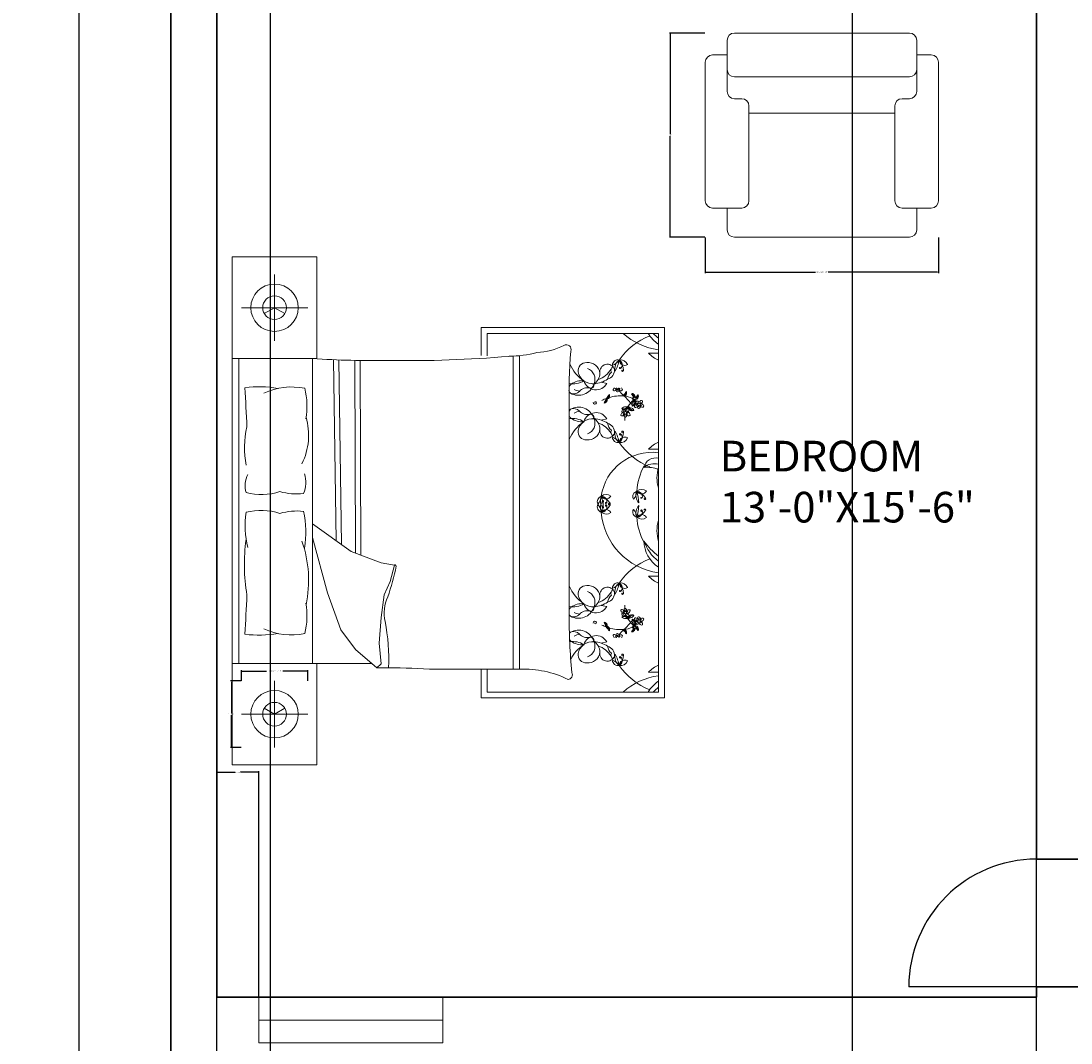
# Model space of a CAD drawing. Units: inches. Extents: x -10 to 502, y -868 to 56.
# Tile 10 of 14: x 6 to 211, y -264 to -64. Entities that reach past the tile are written whole.
import ezdxf

# ---------------------------------------------------------------- set-up
doc = ezdxf.new("R2010")
doc.units = ezdxf.units.IN
doc.header["$MEASUREMENT"] = 0
for name, color, linetype, lineweight in [('A-ANNO-DIMS', 2, 'Continuous', 18), ('A-AREA-IDEN', 7, 'Continuous', 18), ('A-DOOR', 4, 'Continuous', 25), ('A-FURN', 8, 'Continuous', 13), ('A-GLAZ', 162, 'Continuous', 18), ('A-WALL', 7, 'Continuous', 35)]:
    doc.layers.add(name, color=color, linetype=linetype, lineweight=lineweight)
doc.styles.get("Standard").update_dxf_attribs({"font": 'arial.ttf'})
doc.dimstyles.get("Standard").update_dxf_attribs({"dimtxt": 0.18, "dimasz": 0.18, "dimexe": 0.18, "dimexo": 0.0625, "dimgap": 0.09, "dimtad": 0, "dimtih": 1, "dimtoh": 1, "dimdec": 0, "dimzin": 0, "dimdsep": 46, "dimlunit": 3, "dimtxsty": 'Standard', "dimcen": 0.09, "dimadec": 0, "dimazin": 0, "dimtfac": 1, "dimtdec": 0, "dimtofl": 0, "dimtmove": 0, "dimatfit": 3, "dimfxl": 1, "dimtolj": 1, "dimtzin": 0, "dimarcsym": 0})

# ---------------------------------------------------------------- blocks, each defined once
blk = doc.blocks.new('*D2')
at = {"layer": 'A-ANNO-DIMS', "color": 0, "lineweight": -2, "transparency": 16777216}
for p, q in [((34.89, 12.15), (16.75, 12.15)), ((16.93, 11.97), (16.93, -376.2)), ((16.93, -770.67), (16.93, -382.51)), ((34.89, -770.85), (16.75, -770.85))]:
    blk.add_line(p, q, dxfattribs=at)
at = {"layer": 'A-ANNO-DIMS', "color": 0, "transparency": 16777216}
for points in [[(16.9, 11.97), (16.96, 11.97), (16.93, 12.15)], [(16.9, -770.67), (16.96, -770.67), (16.93, -770.85)]]:
    blk.add_solid(points, dxfattribs=at)
at = {"layer": 'Defpoints', "color": 0, "transparency": 16777216}
for p in [(34.95, 12.15), (16.93, -770.85), (34.95, -770.85)]:
    blk.add_point(p, dxfattribs=at)
at = {"layer": 'A-ANNO-DIMS', "color": 0, "transparency": 16777216, "insert": (16.93, -379.35), "char_height": 6, "attachment_point": 5}
blk.add_mtext('\\A1;65\'-3"', dxfattribs=at)
blk = doc.blocks.new('A$C14264F02')
at = {"color": 0}
for p, q in [((0.1, 0.7), (0.7, 0.7)), ((0.1, 0.7), (0.7, 0.7)), ((0.075, 0.625), (0.075, 0.675)), ((0.075, 0.625), (0.075, 0.675)), ((0.725, 0.675), (0.725, 0.575)), ((0.725, 0.675), (0.725, 0.625)), ((0.075, 0.625), (0.025, 0.625)), ((0.025, 0.625), (0.075, 0.625)), ((0.075, 0.575), (0.075, 0.625)), ((0.725, 0.625), (0.775, 0.625)), ((0.725, 0.625), (0.775, 0.625)), ((0, 0.125), (0, 0.6)), ((0, 0.125), (0, 0.6)), ((0.8, 0.6), (0.8, 0.125)), ((0.8, 0.6), (0.8, 0.125)), ((0.075, 0.575), (0.075, 0.5)), ((0.7, 0.55), (0.1, 0.55)), ((0.725, 0.5), (0.725, 0.575)), ((0.1, 0.475), (0.125, 0.475)), ((0.675, 0.475), (0.7, 0.475)), ((0.15, 0.45), (0.15, 0.125)), ((0.65, 0.125), (0.65, 0.45)), ((0.65, 0.425), (0.15, 0.425)), ((0.075, 0.1), (0.025, 0.1)), ((0.075, 0.1), (0.025, 0.1)), ((0.075, 0.025), (0.075, 0.1)), ((0.125, 0.1), (0.075, 0.1)), ((0.775, 0.1), (0.675, 0.1)), ((0.775, 0.1), (0.725, 0.1)), ((0.725, 0.1), (0.725, 0.025)), ((0.7, 0), (0.1, 0))]:
    blk.add_line(p, q, dxfattribs=at)
for centre, start, end in [((0.1, 0.675), 90, 180), ((0.1, 0.675), 90, 180), ((0.7, 0.675), 0, 90), ((0.7, 0.675), 360, 90), ((0.025, 0.6), 90, 180), ((0.025, 0.6), 90, 180), ((0.775, 0.6), 360, 90), ((0.775, 0.6), 0, 90), ((0.1, 0.575), 180, 270), ((0.7, 0.575), 270, 0), ((0.1, 0.5), 180, 270), ((0.125, 0.45), 0, 90), ((0.675, 0.45), 90, 180), ((0.7, 0.5), 270, 360), ((0.025, 0.125), 180, 270), ((0.025, 0.125), 180, 270), ((0.125, 0.125), 270, 360), ((0.675, 0.125), 180, 270), ((0.775, 0.125), 270, 360), ((0.775, 0.125), 270, 360), ((0.1, 0.025), 180, 270), ((0.7, 0.025), 270, 360)]:
    blk.add_arc(centre, 0.025, start, end, dxfattribs=at)
blk = doc.blocks.new('WIN-36IN')
for p, q in [((0, 9), (36, 9)), ((0, 0), (0, 9)), ((36, 9), (36, 0)), ((0, 4.5), (36, 4.5)), ((36, 0), (0, 0))]:
    blk.add_line(p, q)
blk = doc.blocks.new('DOOR-SWING-25IN')
blk.add_line((25, 0), (0, 0))
blk.add_arc((25, 0), 25, 90, 180)
blk = doc.blocks.new('LAMP-BEDSIDE-SMALL')
for p, q in [((6.5, 0), (6.5, 13)), ((13, 6.5), (0, 6.5))]:
    blk.add_line(p, q)
for points in [[(6.5, 6.5), (4.49, 5.34)], [(6.5, 6.5), (8.51, 5.34)]]:
    blk.add_lwpolyline(points)
for radius in [4.64, 2.32]:
    blk.add_circle((6.5, 6.5), radius)
blk = doc.blocks.new('*D35')
at = {"layer": 'A-ANNO-DIMS', "color": 0, "lineweight": -2, "transparency": 16777216}
for p, q in [((139.59, -106.11), (139.59, -113.08)), ((185.27, -106.11), (185.27, -113.08)), ((139.77, -112.9), (161.18, -112.9)), ((185.09, -112.9), (163.68, -112.9))]:
    blk.add_line(p, q, dxfattribs=at)
at = {"layer": 'A-ANNO-DIMS', "color": 0, "transparency": 16777216}
for points in [[(139.77, -112.87), (139.77, -112.93), (139.59, -112.9)], [(185.09, -112.87), (185.09, -112.93), (185.27, -112.9)]]:
    blk.add_solid(points, dxfattribs=at)
at = {"layer": 'Defpoints', "color": 0, "transparency": 16777216}
for p in [(139.59, -106.05), (185.27, -106.05), (139.59, -112.9)]:
    blk.add_point(p, dxfattribs=at)
at = {"layer": 'A-ANNO-DIMS', "color": 0, "transparency": 16777216, "insert": (162.43, -112.9), "char_height": 0.18, "attachment_point": 5}
blk.add_mtext('\\A1;ARMCHAIR 3\'-9 1/2"', dxfattribs=at)
blk = doc.blocks.new('*D36')
at = {"layer": 'A-ANNO-DIMS', "color": 0, "lineweight": -2, "transparency": 16777216}
for p, q in [((139.53, -66.07), (132.56, -66.07)), ((132.74, -66.25), (132.74, -85.88)), ((132.74, -105.87), (132.74, -86.24)), ((139.53, -106.05), (132.56, -106.05))]:
    blk.add_line(p, q, dxfattribs=at)
at = {"layer": 'A-ANNO-DIMS', "color": 0, "transparency": 16777216}
for points in [[(132.71, -66.25), (132.77, -66.25), (132.74, -66.07)], [(132.71, -105.87), (132.77, -105.87), (132.74, -106.05)]]:
    blk.add_solid(points, dxfattribs=at)
at = {"layer": 'Defpoints', "color": 0, "transparency": 16777216}
for p in [(132.74, -66.07), (139.59, -66.07), (139.59, -106.05)]:
    blk.add_point(p, dxfattribs=at)
at = {"layer": 'A-ANNO-DIMS', "color": 0, "transparency": 16777216, "insert": (132.74, -86.06), "char_height": 0.18, "attachment_point": 5}
blk.add_mtext('\\A1;3\'-4"', dxfattribs=at)
blk = doc.blocks.new('*D43')
at = {"layer": 'A-ANNO-DIMS', "color": 0, "lineweight": -2, "transparency": 16777216}
for p, q in [((48.76, -192.9), (48.76, -190.83)), ((48.94, -191.01), (53.66, -191.01)), ((61.58, -191.01), (56.86, -191.01)), ((61.76, -192.9), (61.76, -190.83))]:
    blk.add_line(p, q, dxfattribs=at)
at = {"layer": 'A-ANNO-DIMS', "color": 0, "transparency": 16777216}
for points in [[(48.94, -190.98), (48.94, -191.04), (48.76, -191.01)], [(61.58, -190.98), (61.58, -191.04), (61.76, -191.01)]]:
    blk.add_solid(points, dxfattribs=at)
at = {"layer": 'Defpoints', "color": 0, "transparency": 16777216}
for p in [(48.76, -191.01), (48.76, -192.96), (61.76, -192.96)]:
    blk.add_point(p, dxfattribs=at)
at = {"layer": 'A-ANNO-DIMS', "color": 0, "transparency": 16777216, "insert": (55.26, -191.01), "char_height": 0.18, "attachment_point": 5}
blk.add_mtext('\\A1;BEDSIDE LAMP 1\'-1" TYP.', dxfattribs=at)
blk = doc.blocks.new('*D44')
at = {"layer": 'A-ANNO-DIMS', "color": 0, "lineweight": -2, "transparency": 16777216}
for p, q in [((48.7, -192.96), (46.63, -192.96)), ((46.81, -193.14), (46.81, -199.28)), ((46.81, -205.78), (46.81, -199.64)), ((48.7, -205.96), (46.63, -205.96))]:
    blk.add_line(p, q, dxfattribs=at)
at = {"layer": 'A-ANNO-DIMS', "color": 0, "transparency": 16777216}
for points in [[(46.78, -193.14), (46.84, -193.14), (46.81, -192.96)], [(46.78, -205.78), (46.84, -205.78), (46.81, -205.96)]]:
    blk.add_solid(points, dxfattribs=at)
at = {"layer": 'Defpoints', "color": 0, "transparency": 16777216}
for p in [(48.76, -192.96), (46.81, -205.96), (48.76, -205.96)]:
    blk.add_point(p, dxfattribs=at)
at = {"layer": 'A-ANNO-DIMS', "color": 0, "transparency": 16777216, "insert": (46.81, -199.46), "char_height": 0.18, "attachment_point": 5}
blk.add_mtext('\\A1;1\'-1" TYP.', dxfattribs=at)
blk = doc.blocks.new('*D60')
at = {"layer": 'A-ANNO-DIMS', "color": 0, "lineweight": -2, "transparency": 16777216}
for p, q in [((168.45, -332.79), (168.45, 56.38)), ((168.63, 56.2), (186.12, 56.2)), ((204.27, 56.2), (186.78, 56.2)), ((204.45, -332.79), (204.45, 56.38))]:
    blk.add_line(p, q, dxfattribs=at)
at = {"layer": 'A-ANNO-DIMS', "color": 0, "transparency": 16777216}
for points in [[(168.63, 56.23), (168.63, 56.17), (168.45, 56.2)], [(204.27, 56.23), (204.27, 56.17), (204.45, 56.2)]]:
    blk.add_solid(points, dxfattribs=at)
at = {"layer": 'Defpoints', "color": 0, "transparency": 16777216}
for p in [(204.45, 56.2), (168.45, -332.85), (204.45, -332.85)]:
    blk.add_point(p, dxfattribs=at)
at = {"layer": 'A-ANNO-DIMS', "color": 0, "transparency": 16777216, "insert": (186.45, 56.2), "char_height": 0.18, "attachment_point": 5}
blk.add_mtext('\\A1;3\'-0"', dxfattribs=at)
blk = doc.blocks.new('*D61')
at = {"layer": 'A-ANNO-DIMS', "color": 0, "lineweight": -2, "transparency": 16777216}
for p, q in [((43.95, -254.79), (43.95, -210.62)), ((44.13, -210.8), (47.54, -210.8)), ((52.02, -210.8), (48.61, -210.8)), ((52.2, -254.79), (52.2, -210.62))]:
    blk.add_line(p, q, dxfattribs=at)
at = {"layer": 'A-ANNO-DIMS', "color": 0, "transparency": 16777216}
for points in [[(44.13, -210.77), (44.13, -210.83), (43.95, -210.8)], [(52.02, -210.77), (52.02, -210.83), (52.2, -210.8)]]:
    blk.add_solid(points, dxfattribs=at)
at = {"layer": 'Defpoints', "color": 0, "transparency": 16777216}
for p in [(52.2, -210.8), (43.95, -254.85), (52.2, -254.85)]:
    blk.add_point(p, dxfattribs=at)
at = {"layer": 'A-ANNO-DIMS', "color": 0, "transparency": 16777216, "insert": (48.08, -210.8), "char_height": 0.18, "attachment_point": 5}
blk.add_mtext('\\A1;0\'-8 1/2"', dxfattribs=at)
blk = doc.blocks.new('*D64')
at = {"layer": 'A-ANNO-DIMS', "color": 0, "lineweight": -2, "transparency": 16777216}
for p, q in [((43.95, -332.79), (43.95, 56.38)), ((44.13, 56.2), (48.59, 56.2)), ((54.27, 56.2), (49.81, 56.2)), ((54.45, -332.79), (54.45, 56.38))]:
    blk.add_line(p, q, dxfattribs=at)
at = {"layer": 'A-ANNO-DIMS', "color": 0, "transparency": 16777216}
for points in [[(44.13, 56.23), (44.13, 56.17), (43.95, 56.2)], [(54.27, 56.23), (54.27, 56.17), (54.45, 56.2)]]:
    blk.add_solid(points, dxfattribs=at)
at = {"layer": 'Defpoints', "color": 0, "transparency": 16777216}
for p in [(54.45, 56.2), (43.95, -332.85), (54.45, -332.85)]:
    blk.add_point(p, dxfattribs=at)
at = {"layer": 'A-ANNO-DIMS', "color": 0, "transparency": 16777216, "insert": (49.2, 56.2), "char_height": 0.18, "attachment_point": 5}
blk.add_mtext('\\A1;0\'-10 1/2"', dxfattribs=at)

msp = doc.modelspace()

# ---------------------------------------------------------------- linework, layer by layer
at = {"layer": 'A-FURN'}
for p, q in [((46.97, -209.41), (46.97, -109.91)), ((95.74, -129.25), (95.74, -123.74)), ((95.74, -123.74), (131.59, -123.74)), ((96.9, -124.89), (96.9, -129.28)), ((130.43, -124.89), (96.9, -124.89)), ((130.43, -195.12), (130.43, -124.89)), ((131.59, -123.74), (131.59, -196.28)), ((101.95, -129.36), (101.95, -190.66)), ((103.19, -129.26), (103.19, -190.66)), ((48.24, -129.81), (48.24, -189.51)), ((62.69, -189.51), (62.69, -129.81)), ((66.82, -130.08), (67.32, -165.5)), ((67.85, -130.11), (68.36, -166.25)), ((70.98, -130.17), (71.13, -167.95)), ((72, -130.16), (72.16, -168.34)), ((120.35, -134.69), (119.22, -134.47)), ((112.96, -139.46), (112.96, -179.86)), ((120.35, -141.65), (119.22, -141.87)), ((62.69, -162.18), (70.28, -167.63)), ((65.65, -175.69), (62.69, -164.84)), ((70.28, -167.63), (76.12, -169.84)), ((76.12, -169.84), (78.74, -170.25)), ((78.74, -170.25), (77.93, -173.47)), ((77.93, -173.47), (76.73, -176.09)), ((68.27, -182.94), (65.65, -175.69)), ((76.73, -176.09), (76.12, -180.53)), ((120.35, -178.37), (119.22, -178.15)), ((76.12, -180.53), (75.72, -185.56)), ((71.09, -186.77), (68.27, -182.94)), ((75.32, -190.4), (71.09, -186.77)), ((75.72, -185.56), (76.12, -189.6)), ((120.35, -185.32), (119.22, -185.54)), ((46.97, -189.51), (74.28, -189.51)), ((76.12, -189.6), (75.32, -190.4)), ((95.74, -196.28), (95.74, -190.65)), ((96.9, -190.65), (96.9, -195.12)), ((96.9, -195.12), (130.43, -195.12)), ((131.59, -196.28), (95.74, -196.28))]:
    msp.add_line(p, q, dxfattribs=at)
for points in [[(46.97, -129.81), (63.55, -129.81), (63.55, -109.91), (46.97, -109.91)], [(63.55, -189.51), (63.55, -209.41), (46.97, -209.41)]]:
    msp.add_lwpolyline(points, dxfattribs=at)
for points in [[(101.17, -129.38, 0.056112), (106.64, -128.66, 0.095341), (111.91, -127.26)], [(49.45, -135.52, -0.074897), (55.95, -135.65, 0.472817)], [(56.31, -155.88, -0.14099), (49.68, -156.08, -0.235245)], [(56.31, -160.13, 0.14099), (49.68, -159.93, 0.235245)], [(49.45, -183.8, 0.074897), (55.95, -183.67, -0.472817)], [(84.43, -190.61, 0.001242), (103.31, -190.66, -0.127202), (112.72, -192.65)]]:
    msp.add_lwpolyline(points, format="xyb", dxfattribs=at)
for centre in [(126.62, -138.79), (123.95, -140.44), (123.95, -179.57), (126.62, -181.23)]:
    msp.add_circle(centre, 0.253, dxfattribs=at)
for centre, radius, start, end in [((133.47, -137.45), 12.99, 111.4092, 145.6135), ((132.18, -115.22), 12.99, 228.1144, 262.255), ((133.92, -121.73), 6.33, 209.8884, 236.5383), ((135.11, -119.46), 7.89, 223.5186, 233.6964), ((112.42, -128.02), 0.907, 336.5219, 123.8264), ((81.35, 102.99), 233.22, 269.1145, 274.8735), ((209.74, -136.41), 96.82, 175.2402, 181.8035), ((132.46, -125.28), 5.28, 221.0454, 247.4453), ((129.62, -110.81), 17.98, 266.3481, 272.5919), ((74.85, 48.57), 178.79, 266.1, 270.9282), ((119.97, -127.89), 7.53, 203.6453, 236.3329), ((116.35, -132.28), 1.68, 88.9462, 185.5144), ((116.6, -132.97), 2.38, 7.1143, 95.0551), ((120.43, -132.42), 1.49, 19.1312, 189.736), ((122.04, -132.11), 0.915, 126.7319, 206.0245), ((122.49, -131.15), 1.08, 76.272, 177.0484), ((120.85, -128.95), 2.22, 284.7031, 328.6173), ((123.95, -131.77), 2.05, 125.7657, 194.5347), ((113.87, -128.14), 9.09, 332.8176, 347.4827), ((123.05, -131.52), 1.44, 20.9613, 102.2885), ((123.83, -130.08), 1.09, 181.7131, 301.5367), ((120.27, -132.27), 3.29, 2.0648, 41.1598), ((122.25, -131.05), 1.06, 316.2238, 62.3173), ((117.6, -131.76), 2.99, 193.079, 274.7067), ((115.69, -133.9), 2.31, 338.5779, 68.4181), ((116.07, -132.55), 2.89, 305.9599, 357.6409), ((117.14, -129.46), 4.7, 288.2955, 328.7386), ((119.98, -132.06), 1.86, 285.6955, 4.031), ((122.46, -134.07), 1.99, 128.4175, 173.8338), ((122.87, -131.67), 0.0847, 20.2667, 316.2271), ((123.4, -132.16), 0.161, 168.5166, 2.0648), ((123.31, -132.14), 0.0784, 52.0591, 168.5166), ((-897.48, -190.37), 948.52, 2.85022, 3.31479), ((58.56, -148.2), 12.82, 78.2417, 114.8684), ((48.28, -139.07), 13.33, 348.9631, 14.8961), ((114.06, -135.76), 1.2, 127.675, 162.5814), ((113.7, -130.65), 4.12, 259.249, 301.1782), ((114.77, -133.84), 3.17, 240.8249, 340.7178), ((115.49, -137.98), 3.84, 85.2696, 124.215), ((116.47, -137.59), 2.04, 74.8529, 138.4347), ((118.2, -133.46), 2.47, 196.8663, 330.0915), ((117.16, -135.03), 0.618, 254.8529, 12.6959), ((115.49, -137.98), 3.84, 53.6555, 57.2989), ((117.52, -129.41), 5.34, 273.4924, 303.7117), ((122.05, -135.88), 0.423, 127.3642, 168.4363), ((122.21, -135.83), 0.242, 88.1325, 178.8919), ((122.45, -135.53), 0.253, 183.2768, 356.7232), ((122.36, -136.33), 0.769, 42.3896, 66.5724), ((122.91, -135.88), 0.418, 10.9597, 52.2379), ((114.06, -135.76), 1.2, 196.6343, 225.5483), ((113.83, -135.25), 1.49, 246.1646, 318.4347), ((115.35, -133.37), 2.86, 240.0851, 262.564), ((123.11, -145.35), 8.24, 110.1059, 116.9968), ((120.29, -137.93), 0.203, 83.9457, 185.6216), ((119.48, -137.74), 0.834, 328.836, 0.8141), ((119.91, -137.98), 0.478, 306.5232, 32.4668), ((120.48, -137.61), 0.203, 112.5583, 214.2343), ((120.34, -137.25), 0.478, 265.7131, 351.6568), ((119.93, -136.98), 0.834, 297.3659, 329.344), ((119.29, -136.27), 1.6, 313.6929, 321.7899), ((121.06, -137.36), 0.522, 115.5379, 168.6744), ((119.29, -136.61), 1.57, 329.344, 349.7412), ((123.11, -145.35), 8.24, 86.1723, 106.4158), ((118.03, -136.97), 2.81, 352.8698, 1.6736), ((121.75, -135.96), 0.196, 125.0752, 284.7644), ((121.72, -135.54), 0.609, 277.4968, 341.2737), ((122.69, -136.08), 0.524, 136.3462, 189.6513), ((122.39, -136.13), 0.218, 189.6513, 312.3208), ((123.24, -135.98), 0.83, 164.2829, 186.9148), ((122.26, -135.99), 0.415, 312.3208, 40.2111), ((123.14, -135.52), 0.589, 201.6382, 274.947), ((130.12, -130.24), 9.45, 217.9541, 226.8459), ((123.17, -135.92), 0.194, 274.947, 37.5263), ((123.82, -137.02), 0.203, 112.5583, 214.2343), ((123.69, -136.66), 0.478, 265.7131, 351.6568), ((123.27, -136.39), 0.834, 297.3659, 329.344), ((123.31, -141.25), 4.13, 60.7959, 85.244), ((114.52, -147.2), 13.6, 37.8256, 47.7588), ((122.64, -135.67), 1.6, 313.6929, 321.7899), ((124.41, -136.77), 0.522, 115.5379, 168.6744), ((122.64, -136.01), 1.57, 329.344, 349.7412), ((121.38, -136.38), 2.81, 352.8698, 1.6736), ((125.33, -136.94), 0.283, 33.0979, 123.1364), ((119.09, -140.93), 7.4, 31.1156, 34.8118), ((124.92, -137.43), 0.766, 2.3172, 70.5201), ((125.55, -137.62), 0.221, 135.7354, 318.1297), ((125.18, -137.26), 0.293, 315.7354, 31.1156), ((125.72, -137.61), 0.221, 68.2452, 250.6395), ((125.21, -137.34), 0.66, 352.6008, 57.1845), ((127.56, -141.77), 4.41, 111.7087, 116.2181), ((125.84, -137.19), 0.66, 252.8042, 349.6943), ((125.91, -137.14), 0.293, 248.2452, 323.6254), ((125.65, -136.96), 0.766, 291.7087, 3.0299), ((120.18, -132.92), 7.4, 323.6254, 327.3216), ((126.25, -137.15), 0.283, 325.6077, 55.6462), ((114.06, -140.59), 1.2, 134.4517, 156.7144), ((114.77, -142.5), 3.17, 19.2822, 119.1751), ((113.83, -141.09), 1.49, 41.5653, 113.8354), ((117.98, -138.44), 0.312, 169.5864, 349.5616), ((118.1, -138.46), 0.192, 349.5616, 167.2949), ((120.34, -138.56), 0.522, 129.5056, 182.6421), ((118.84, -137.35), 1.57, 308.4388, 328.836), ((118.57, -136.07), 2.81, 296.5064, 305.3102), ((118.55, -137.52), 1.6, 336.3901, 344.4871), ((123.57, -138.5), 1.16, 253.6301, 325.4631), ((123.9, -140.11), 0.817, 82.0748, 142.6895), ((123.81, -138.98), 0.839, 228.342, 274.9894), ((123.83, -139.12), 0.702, 273.8774, 357.1501), ((124.72, -140.38), 0.799, 121.9501, 165.2442), ((124.11, -138.62), 0.68, 262.0748, 308.2393), ((124.14, -139.93), 0.5, 278.5614, 22.5914), ((128.8, -141.67), 4.96, 156.1523, 156.9499), ((124.43, -139.91), 0.251, 44.3732, 121.9501), ((125.2, -139.32), 0.702, 181.4625, 249.4747), ((128.8, -141.67), 4.96, 130.182, 149.456), ((125.08, -138.77), 0.68, 215.1128, 261.2773), ((125.63, -138.8), 1.16, 197.889, 269.722), ((124.86, -140.25), 0.817, 20.6625, 81.2773), ((126.07, -138.85), 0.817, 139.3812, 199.9959), ((124.55, -138.26), 1.16, 310.9365, 22.7695), ((125.08, -138.32), 0.839, 285.6484, 332.2957), ((124.94, -137.88), 0.68, 319.3812, 5.5456), ((123.31, -141.25), 4.13, 47.5083, 55.9967), ((125.21, -138.37), 0.702, 331.1838, 51.6792), ((125.93, -139.21), 0.196, 125.0752, 284.7644), ((126.23, -139.14), 0.423, 93.635, 168.4363), ((126.18, -138.47), 0.248, 138.2946, 276.2474), ((125.9, -138.8), 0.609, 277.4968, 341.2737), ((126.27, -138.51), 0.346, 358.5719, 143.8954), ((126.38, -139.08), 0.242, 88.1325, 178.8919), ((126.47, -138.23), 0.349, 208.8493, 269.9355), ((126.17, -138.32), 0.399, 274.2123, 318.1587), ((126.87, -139.34), 0.524, 136.3462, 189.6513), ((126.57, -139.39), 0.218, 189.6513, 312.3208), ((127.41, -139.24), 0.83, 164.2829, 186.9148), ((127.39, -138.72), 0.799, 121.9501, 165.2442), ((126.44, -139.24), 0.415, 312.3208, 40.2111), ((127.31, -138.78), 0.589, 201.6382, 274.947), ((126.84, -138.41), 0.168, 262.868, 7.094), ((126.53, -139.58), 0.769, 42.3896, 66.5724), ((126.82, -138.27), 0.5, 278.5614, 22.5914), ((127.09, -139.13), 0.418, 10.9597, 118.7804), ((127.1, -138.25), 0.251, 44.3732, 121.9501), ((127.35, -139.17), 0.194, 274.947, 37.5263), ((49.26, -144.83), 12.67, 333.8761, 16.1746), ((114.06, -140.59), 1.2, 203.2856, 232.325), ((113.7, -145.69), 4.12, 58.8218, 100.2867), ((115.49, -138.36), 3.84, 235.785, 274.7304), ((115.35, -142.98), 2.86, 97.436, 119.9149), ((117.6, -144.58), 2.99, 85.2933, 166.921), ((116.47, -138.75), 2.04, 221.5653, 285.1471), ((118.2, -142.88), 2.47, 29.9085, 163.1337), ((115.69, -142.44), 2.31, 291.5819, 21.4221), ((117.16, -141.32), 0.618, 347.3041, 105.1471), ((115.49, -138.36), 3.84, 302.7011, 306.3445), ((116.07, -143.79), 2.89, 2.3591, 54.0401), ((117.52, -146.93), 5.34, 56.2883, 86.5076), ((123.26, -140.87), 0.196, 125.0752, 284.7644), ((123.56, -140.79), 0.423, 93.635, 168.4363), ((123.51, -140.13), 0.248, 138.2946, 276.2474), ((123.23, -140.45), 0.609, 277.4968, 341.2737), ((123.6, -140.16), 0.346, 358.5719, 143.8954), ((123.71, -140.74), 0.242, 88.1325, 178.8919), ((123.8, -139.89), 0.349, 208.8493, 269.9355), ((123.5, -139.97), 0.399, 274.2123, 318.1587), ((124.2, -141), 0.524, 136.3462, 189.6513), ((123.9, -141.05), 0.218, 189.6513, 312.3208), ((128.8, -141.67), 4.96, 175.2415, 182.8929), ((124.74, -140.9), 0.83, 164.2829, 186.9148), ((123.77, -140.9), 0.415, 312.3208, 40.2111), ((124.64, -140.43), 0.589, 201.6382, 274.947), ((124.17, -140.07), 0.168, 262.868, 7.094), ((123.86, -141.24), 0.769, 42.3896, 66.5724), ((124.42, -140.79), 0.418, 10.9597, 118.7804), ((124.68, -140.83), 0.194, 274.947, 37.5263), ((125.27, -139.2), 0.839, 248.3627, 295.0101), ((66.86, -147.33), 17.49, 166.3427, 191.1841), ((119.97, -148.45), 7.53, 123.6671, 158.5059), ((116.35, -144.07), 1.68, 174.4856, 271.0538), ((116.6, -143.38), 2.38, 264.9449, 352.8857), ((117.14, -146.89), 4.7, 31.2614, 71.7045), ((120.43, -143.92), 1.49, 170.264, 340.8688), ((122.46, -142.27), 1.99, 186.1662, 231.5825), ((119.98, -144.28), 1.86, 355.969, 74.3045), ((122.04, -144.23), 0.915, 153.9755, 233.2681), ((122.49, -145.19), 1.08, 182.9516, 283.728), ((120.85, -147.39), 2.22, 31.3827, 75.2969), ((123.95, -144.57), 2.05, 165.4653, 234.2343), ((113.87, -148.21), 9.09, 12.5173, 27.1824), ((120.27, -144.07), 3.29, 318.8402, 357.9352), ((122.25, -145.29), 1.06, 297.6827, 43.7762), ((123.83, -146.27), 1.09, 58.4633, 178.2869), ((123.05, -144.83), 1.44, 257.7115, 339.0387), ((122.92, -144.66), 0.141, 43.7762, 339.7183), ((123.4, -144.19), 0.161, 357.9352, 191.4834), ((123.31, -144.2), 0.0784, 191.4834, 307.9409), ((133.47, -138.9), 12.99, 214.3865, 248.5908), ((132.46, -151.06), 5.28, 112.5547, 138.9546), ((129.62, -165.53), 17.98, 87.4081, 93.6519), ((129.18, -158.23), 10.06, 82.8636, 171.8197), ((129.88, -151.59), 2.33, 76.3898, 169.0739), ((139.14, -156.82), 12.99, 152.5854, 175.5377), ((129.56, -153.35), 2.95, 72.8609, 131.9049), ((128.27, -156.93), 5.82, 68.117, 96.6195), ((137.27, -153.18), 7.14, 162.9798, 196.4569), ((54.41, -154.71), 4.92, 153.3437, 196.1026), ((56.13, -154.05), 5.27, 335.0183, 18.5407), ((59.64, -144.15), 12.19, 254.1707, 275.9871), ((126.49, -156.84), 1.08, 106.1963, 206.9726), ((123.97, -155.75), 2.22, 314.6273, 358.5415), ((128.06, -156.65), 2.05, 155.6899, 224.4589), ((127.16, -156.87), 1.44, 50.8855, 132.2127), ((127.11, -155.24), 1.09, 211.6373, 331.4609), ((126.23, -156.87), 1.06, 346.148, 92.2415), ((125.12, -158.91), 3.29, 31.989, 71.0841), ((117.52, -158.52), 9.09, 2.7418, 17.407), ((140.95, -156.01), 10.57, 174.3643, 175.6213), ((148.19, -161.58), 18.88, 160.0972, 160.2783), ((119.53, -157.83), 1.08, 106.1963, 206.9726), ((117.01, -156.74), 2.22, 314.6273, 358.5415), ((121.1, -157.65), 2.05, 155.6899, 224.4589), ((121.1, -159.05), 2.05, 135.5411, 204.3101), ((120.2, -157.87), 1.44, 50.8855, 132.2127), ((120.15, -156.23), 1.09, 211.6373, 331.4609), ((119.27, -157.86), 1.06, 346.148, 92.2415), ((118.17, -159.91), 3.29, 31.989, 71.0841), ((110.56, -159.52), 9.09, 2.7418, 17.407), ((110.56, -157.18), 9.09, 342.593, 357.2582), ((120.11, -158.1), 0.0847, 50.1909, 346.0209), ((120.82, -158.25), 0.161, 198.4408, 31.989), ((120.74, -158.28), 0.0784, 81.9833, 198.4408), ((120.82, -158.44), 0.161, 328.011, 161.5592), ((127.07, -157.1), 0.0847, 50.1909, 346.0209), ((127.78, -157.26), 0.161, 198.4408, 31.989), ((127.7, -157.28), 0.0784, 81.9833, 198.4408), ((67.22, -162.54), 17.73, 171.5249, 193.96), ((59.64, -171.86), 12.19, 84.0129, 105.8293), ((43.85, -163.86), 17.55, 349.8617, 13.6238), ((119.53, -158.86), 1.08, 153.0274, 253.8037), ((117.01, -159.95), 2.22, 1.4585, 45.3727), ((118.17, -156.79), 3.29, 288.9159, 328.011), ((119.27, -158.84), 1.06, 267.7585, 13.852), ((120.15, -160.47), 1.09, 28.5391, 148.3627), ((120.2, -158.83), 1.44, 227.7873, 309.1145), ((132.18, -158.89), 12.99, 184.4623, 262.255), ((120.17, -158.61), 0.141, 13.852, 309.9245), ((120.74, -158.42), 0.0784, 161.5592, 278.0167), ((126.49, -159.86), 1.08, 153.0274, 253.8037), ((123.97, -160.95), 2.22, 1.4585, 45.3727), ((128.06, -160.05), 2.05, 135.5411, 204.3101), ((117.52, -158.17), 9.09, 342.593, 357.2582), ((125.12, -157.78), 3.29, 288.9159, 328.011), ((126.23, -159.83), 1.06, 267.7585, 13.852), ((127.13, -159.61), 0.141, 13.852, 309.9245), ((127.78, -159.44), 0.161, 328.011, 161.5592), ((127.7, -159.41), 0.0784, 161.5592, 278.0167), ((127.11, -161.46), 1.09, 28.5391, 148.3627), ((127.16, -159.82), 1.44, 227.7873, 309.1145), ((139.14, -159.88), 12.99, 184.4623, 207.4146), ((137.27, -163.51), 7.14, 163.5431, 197.0202), ((140.95, -160.68), 10.57, 184.3787, 185.6357), ((148.19, -155.12), 18.88, 199.7217, 199.9028), ((85.45, -170.16), 36.09, 172.2196, 189.497), ((38.8, -173.23), 23.13, 348.0397, 19.2615), ((133.92, -165.4), 6.33, 181.272, 236.5383), ((137.32, -158.98), 11.74, 214.0123, 234.053), ((135.11, -163.13), 7.89, 197.8504, 233.6964), ((41.14, -163.34), 38.59, 340.1194, 349.3383), ((78.82, -170.47), 0.24, 358.8623, 109.7536), ((133.47, -181.12), 12.99, 111.4092, 145.6135), ((129.62, -154.48), 17.98, 266.3481, 272.5919), ((132.46, -168.95), 5.28, 221.0454, 247.4453), ((119.97, -171.56), 7.53, 201.4941, 236.3329), ((116.35, -175.95), 1.68, 88.9462, 185.5144), ((116.6, -176.64), 2.38, 7.1143, 95.0551), ((120.43, -176.09), 1.49, 19.1312, 189.736), ((122.49, -174.82), 1.08, 76.272, 177.0484), ((120.85, -172.62), 2.22, 284.7031, 328.6173), ((123.95, -175.44), 2.05, 125.7657, 194.5347), ((113.87, -171.81), 9.09, 332.8176, 347.4827), ((123.05, -175.19), 1.44, 20.9613, 102.2885), ((122.25, -174.72), 1.06, 316.2238, 62.3173), ((120.27, -175.94), 3.29, 2.0648, 41.1598), ((123.83, -173.75), 1.09, 181.7131, 301.5367), ((-897.48, -128.95), 948.52, 356.68521, 357.14978), ((84.84, -179.72), 8.1, 156.2616, 191.3392), ((117.6, -175.43), 2.99, 193.079, 274.7067), ((115.69, -177.57), 2.31, 338.5779, 68.4181), ((116.07, -176.22), 2.89, 305.9599, 357.6409), ((117.14, -173.13), 4.7, 288.2955, 328.7386), ((119.98, -175.73), 1.86, 285.6955, 4.031), ((122.46, -177.74), 1.99, 128.4175, 173.8338), ((122.04, -175.78), 0.915, 126.7319, 206.0245), ((122.87, -175.34), 0.0847, 20.2667, 316.2271), ((123.4, -175.83), 0.161, 168.5166, 2.0648), ((123.31, -175.81), 0.0784, 52.0591, 168.5166), ((48.28, -180.25), 13.33, 345.1039, 11.0369), ((113.7, -174.32), 4.12, 259.7133, 301.1782), ((114.06, -179.43), 1.2, 127.675, 156.7144), ((114.77, -177.52), 3.17, 240.8249, 340.7178), ((115.49, -181.65), 3.84, 85.2696, 124.215), ((118.2, -177.13), 2.47, 196.8663, 330.0915), ((117.16, -178.7), 0.618, 254.8529, 12.6959), ((115.49, -181.65), 3.84, 53.6555, 57.2989), ((117.52, -173.08), 5.34, 273.4924, 303.7117), ((123.9, -178.97), 0.218, 47.6792, 170.3487), ((128.8, -178.34), 4.96, 177.1071, 184.7585), ((123.77, -179.11), 0.415, 319.7889, 47.6792), ((216.54, -181.05), 103.58, 179.3433, 185.6887), ((114.06, -179.43), 1.2, 203.229, 225.5483), ((113.83, -178.92), 1.49, 246.1646, 318.4347), ((115.35, -177.04), 2.86, 240.0851, 262.564), ((116.47, -181.26), 2.04, 74.8529, 138.4347), ((123.26, -179.14), 0.196, 75.2356, 234.9248), ((123.56, -179.22), 0.423, 191.5637, 266.365), ((123.81, -181.03), 0.839, 85.0106, 131.658), ((123.57, -181.51), 1.16, 34.5369, 106.3699), ((123.9, -179.91), 0.817, 217.3105, 277.9252), ((123.51, -179.89), 0.248, 83.7526, 221.7054), ((123.23, -179.56), 0.609, 18.7263, 82.5032), ((123.6, -179.85), 0.346, 216.1046, 1.4281), ((123.71, -179.28), 0.242, 181.1081, 271.8675), ((123.8, -180.12), 0.349, 90.0645, 151.1507), ((123.5, -180.04), 0.399, 41.8413, 85.7877), ((124.2, -179.02), 0.524, 170.3487, 223.6538), ((123.83, -180.89), 0.702, 2.8499, 86.1226), ((124.74, -179.12), 0.83, 173.0852, 195.7171), ((124.72, -179.64), 0.799, 194.7558, 238.0499), ((124.11, -181.39), 0.68, 51.7607, 97.9252), ((124.64, -179.58), 0.589, 85.053, 158.3618), ((124.17, -179.95), 0.168, 352.906, 97.132), ((123.86, -178.77), 0.769, 293.4276, 317.6104), ((124.42, -179.23), 0.418, 241.2196, 349.0403), ((124.14, -180.09), 0.5, 337.4086, 81.4386), ((128.8, -178.34), 4.96, 203.0501, 203.8477), ((124.43, -180.1), 0.251, 238.0499, 315.6268), ((125.2, -180.69), 0.702, 110.5253, 178.5375), ((125.63, -181.21), 1.16, 90.278, 162.111), ((125.08, -181.25), 0.68, 98.7227, 144.8872), ((128.8, -178.34), 4.96, 210.544, 229.818), ((124.68, -179.19), 0.194, 322.4737, 85.053), ((125.27, -180.82), 0.839, 64.9899, 111.6373), ((124.86, -179.77), 0.817, 278.7227, 339.3375), ((126.07, -181.16), 0.817, 160.0041, 220.6188), ((124.55, -181.76), 1.16, 337.2305, 49.0635), ((125.08, -181.69), 0.839, 27.7043, 74.3516), ((125.93, -180.8), 0.196, 75.2356, 234.9248), ((125.9, -181.22), 0.609, 18.7263, 82.5032), ((126.57, -180.62), 0.218, 47.6792, 170.3487), ((126.87, -180.68), 0.524, 170.3487, 223.6538), ((127.41, -180.78), 0.83, 173.0852, 195.7171), ((126.44, -180.77), 0.415, 319.7889, 47.6792), ((127.31, -181.24), 0.589, 85.053, 158.3618), ((127.35, -180.84), 0.194, 322.4737, 85.053), ((58.56, -171.12), 12.82, 245.1316, 281.7583), ((40.08, -188.7), 37.55, 357.4519, 11.3392), ((117.98, -181.58), 0.312, 10.4384, 190.4136), ((118.1, -181.56), 0.192, 192.7051, 10.4384), ((123.11, -174.66), 8.24, 243.0032, 249.8941), ((118.84, -182.66), 1.57, 31.164, 51.5612), ((120.34, -181.45), 0.522, 177.3579, 230.4944), ((118.57, -183.94), 2.81, 54.6898, 63.4936), ((118.55, -182.5), 1.6, 15.5129, 23.6099), ((120.29, -182.09), 0.203, 174.3784, 276.0543), ((119.91, -182.03), 0.478, 327.5332, 53.4768), ((119.48, -182.28), 0.834, 359.1859, 31.164), ((120.48, -182.4), 0.203, 145.7657, 247.4417), ((120.34, -182.77), 0.478, 8.3432, 94.2869), ((119.93, -183.03), 0.834, 30.656, 62.6341), ((119.29, -183.75), 1.6, 38.2101, 46.3071), ((121.06, -182.66), 0.522, 191.3256, 244.4621), ((119.29, -183.41), 1.57, 10.2588, 30.656), ((123.11, -174.66), 8.24, 253.5842, 273.8277), ((118.03, -183.04), 2.81, 358.3264, 7.1302), ((130.12, -189.77), 9.45, 133.1541, 142.0459), ((123.82, -183), 0.203, 145.7657, 247.4417), ((114.52, -172.82), 13.6, 312.2412, 322.1744), ((123.31, -178.77), 4.13, 274.756, 299.2041), ((123.69, -183.36), 0.478, 8.3432, 94.2869), ((123.27, -183.62), 0.834, 30.656, 62.6341), ((124.92, -182.59), 0.766, 289.4799, 357.6828), ((119.09, -179.08), 7.4, 325.1882, 328.8844), ((125.55, -182.4), 0.221, 41.8703, 224.2646), ((125.18, -182.76), 0.293, 328.8844, 44.2646), ((124.94, -182.14), 0.68, 354.4544, 40.6188), ((125.72, -182.4), 0.221, 109.3605, 291.7548), ((125.21, -182.67), 0.66, 302.8155, 7.3992), ((127.56, -178.24), 4.41, 243.7819, 248.2913), ((123.31, -178.77), 4.13, 304.0033, 312.4917), ((125.21, -181.64), 0.702, 308.3208, 28.8162), ((125.84, -182.82), 0.66, 10.3057, 107.1958), ((125.91, -182.88), 0.293, 36.3746, 111.7548), ((126.23, -180.88), 0.423, 191.5637, 266.365), ((126.18, -181.55), 0.248, 83.7526, 221.7054), ((125.65, -183.06), 0.766, 356.9701, 68.2913), ((126.27, -181.51), 0.346, 216.1046, 1.4281), ((126.38, -180.93), 0.242, 181.1081, 271.8675), ((120.18, -187.09), 7.4, 32.6784, 36.3746), ((126.47, -181.78), 0.349, 90.0645, 151.1507), ((126.17, -181.7), 0.399, 41.8413, 85.7877), ((126.25, -182.86), 0.283, 304.3538, 34.3923), ((127.39, -181.3), 0.799, 194.7558, 238.0499), ((126.84, -181.6), 0.168, 352.906, 97.132), ((126.53, -180.43), 0.769, 293.4276, 317.6104), ((127.09, -180.88), 0.418, 241.2196, 349.0403), ((126.82, -181.74), 0.5, 337.4086, 81.4386), ((127.1, -181.76), 0.251, 238.0499, 315.6268), ((114.06, -184.26), 1.2, 134.4517, 153.558), ((114.06, -184.26), 1.2, 210.0293, 232.325), ((114.77, -186.17), 3.17, 19.2822, 119.1751), ((113.83, -184.76), 1.49, 41.5653, 113.8354), ((115.35, -186.65), 2.86, 97.436, 119.9149), ((116.47, -182.42), 2.04, 221.5653, 285.1471), ((118.2, -186.55), 2.47, 29.9085, 163.1337), ((117.16, -184.99), 0.618, 347.3041, 105.1471), ((121.75, -184.06), 0.196, 75.2356, 234.9248), ((122.05, -184.13), 0.423, 191.5637, 232.6358), ((121.72, -184.47), 0.609, 18.7263, 82.5032), ((122.21, -184.19), 0.242, 181.1081, 271.8675), ((122.69, -183.93), 0.524, 170.3487, 223.6538), ((122.39, -183.88), 0.218, 47.6792, 170.3487), ((122.45, -184.48), 0.253, 3.2768, 176.7232), ((123.24, -184.03), 0.83, 173.0852, 195.7171), ((122.26, -184.02), 0.415, 319.7889, 47.6792), ((123.14, -184.49), 0.589, 85.053, 158.3618), ((122.36, -183.69), 0.769, 293.4276, 317.6104), ((122.91, -184.14), 0.418, 307.7621, 349.0403), ((123.17, -184.1), 0.194, 322.4737, 85.053), ((122.64, -184.34), 1.6, 38.2101, 46.3071), ((124.41, -183.25), 0.522, 191.3256, 244.4621), ((122.64, -184), 1.57, 10.2588, 30.656), ((121.38, -183.64), 2.81, 358.3264, 7.1302), ((125.33, -183.07), 0.283, 236.8636, 326.9021), ((113.7, -189.36), 4.12, 58.8218, 99.1554), ((119.97, -192.12), 7.53, 123.6671, 153.2997), ((115.49, -182.03), 3.84, 235.785, 274.7304), ((117.6, -188.25), 2.99, 85.2933, 166.921), ((115.69, -186.11), 2.31, 291.5819, 21.4221), ((115.49, -182.03), 3.84, 302.7011, 306.3445), ((116.07, -187.46), 2.89, 2.3591, 54.0401), ((117.52, -190.6), 5.34, 56.2883, 86.5076), ((117.14, -190.56), 4.7, 31.2614, 71.7045), ((119.98, -187.95), 1.86, 355.969, 74.3045), ((122.46, -185.94), 1.99, 186.1662, 231.5825), ((116.35, -187.74), 1.68, 174.4856, 271.0538), ((116.6, -187.05), 2.38, 264.9449, 352.8857), ((120.43, -187.6), 1.49, 170.264, 340.8688), ((122.04, -187.9), 0.915, 153.9755, 233.2681), ((120.85, -191.06), 2.22, 31.3827, 75.2969), ((122.49, -188.86), 1.08, 182.9516, 283.728), ((123.95, -188.24), 2.05, 165.4653, 234.2343), ((113.87, -191.88), 9.09, 12.5173, 27.1824), ((120.27, -187.74), 3.29, 318.8402, 357.9352), ((122.25, -188.97), 1.06, 297.6827, 43.7762), ((123.83, -189.94), 1.09, 58.4633, 178.2869), ((123.05, -188.5), 1.44, 257.7115, 339.0387), ((122.92, -188.33), 0.141, 43.7762, 339.7183), ((123.4, -187.86), 0.161, 357.9352, 191.4834), ((123.31, -187.87), 0.0784, 191.4834, 307.9409), ((77.79, -281.63), 91.27, 85.8294, 91.553), ((133.47, -182.57), 12.99, 214.3865, 248.5908), ((132.46, -194.73), 5.28, 112.5547, 138.9546), ((112.65, -191.74), 0.918, 273.98, 27.3412), ((132.18, -204.8), 12.99, 97.745, 131.8856), ((133.92, -198.28), 6.33, 123.4617, 150.1116), ((129.62, -209.21), 17.98, 87.4081, 93.6519), ((135.11, -200.56), 7.89, 126.3036, 136.4814)]:
    msp.add_arc(centre, radius, start, end, dxfattribs=at)
at = {"layer": 'A-WALL'}
for p, q in [((34.95, 12.15), (34.95, -770.85)), ((43.95, -61.35), (43.95, -254.85)), ((204.45, -61.35), (204.45, -227.85)), ((213.45, -227.85), (204.45, -227.85)), ((213.45, -252.85), (204.45, -252.85)), ((204.45, -252.85), (204.45, -254.85)), ((43.95, -254.85), (204.45, -254.85))]:
    msp.add_line(p, q, dxfattribs=at)

# ---------------------------------------------------------------- block references
at = {"layer": 'A-DOOR'}
msp.add_blockref('DOOR-SWING-25IN', (179.45, -252.85), dxfattribs=at)
at = {"layer": 'A-FURN', "ltscale": 0.03, "xscale": -57.10174686868406, "yscale": 57.10174686868406, "zscale": 57.10174686868406}
msp.add_blockref('A$C14264F02', (185.27, -106.05), dxfattribs=at)
at = {"layer": 'A-FURN'}
msp.add_blockref('LAMP-BEDSIDE-SMALL', (48.76, -126.36), dxfattribs=at)
at = {"layer": 'A-FURN', "rotation": 180}
msp.add_blockref('LAMP-BEDSIDE-SMALL', (61.76, -192.96), dxfattribs=at)
at = {"layer": 'A-GLAZ', "rotation": 180}
msp.add_blockref('WIN-36IN', (88.2, -254.85), dxfattribs=at)

# ---------------------------------------------------------------- texts
at = {"layer": 'A-AREA-IDEN', "insert": (142.43, -145.92), "char_height": 6, "attachment_point": 1}
msp.add_mtext('BEDROOM\\P13\'-0"X15\'-6"', dxfattribs=at)

# ---------------------------------------------------------------- dimensions: what is measured, and where the dimension line sits
at = {"layer": 'A-ANNO-DIMS'}
for base, p1, p2, picture, middle in [((54.45, 56.2), (43.95, -332.85), (54.45, -332.85), '*D64', (49.2, 56.2)), ((204.45, 56.2), (168.45, -332.85), (204.45, -332.85), '*D60', (186.45, 56.2))]:
    dim = msp.add_linear_dim(base=base, p1=p1, p2=p2, dimstyle='Standard', override={"dimdec": 1, "dimlfac": 1, "dimrnd": 0, "dimzin": 1, "dimdsep": 46, "dimlunit": 4, "dimfrac": 2}, dxfattribs=at)
    dim.commit()
    dim.dimension.update_dxf_attribs({"geometry": picture, "text_midpoint": middle})
for base, p1, p2, angle, override, picture, middle in [((16.93, -770.85), (34.95, 12.15), (34.95, -770.85), 90, {"dimtxt": 6, "dimclrd": 0, "dimclre": 0, "dimclrt": 0}, '*D2', (16.93, -379.35)), ((132.74, -66.07), (139.59, -106.05), (139.59, -66.07), 90, {"dimdec": 1, "dimlfac": 1, "dimrnd": 0, "dimzin": 1, "dimdsep": 46, "dimlunit": 4, "dimfrac": 2}, '*D36', (132.74, -86.06)), ((52.200916, -210.802737), (43.950916, -254.852737), (52.200916, -254.852737), 0, {"dimdec": 1, "dimlfac": 1, "dimrnd": 0, "dimzin": 1, "dimdsep": 46, "dimlunit": 4, "dimfrac": 2}, '*D61', (48.075916, -210.802737))]:
    dim = msp.add_linear_dim(base=base, p1=p1, p2=p2, angle=angle, dimstyle='Standard', override=override, dxfattribs=at)
    dim.commit()
    dim.dimension.update_dxf_attribs({"geometry": picture, "text_midpoint": middle})
for base, p1, p2, angle, text, picture, middle in [((139.59, -112.9), (185.27, -106.05), (139.59, -106.05), 180, 'ARMCHAIR <>', '*D35', (162.43, -112.9)), ((48.76, -191.01), (61.76, -192.96), (48.76, -192.96), 180, 'BEDSIDE LAMP <> TYP.', '*D43', (55.26, -191.01)), ((46.81, -205.96), (48.76, -192.96), (48.76, -205.96), 270, '<> TYP.', '*D44', (46.81, -199.46))]:
    dim = msp.add_linear_dim(base=base, p1=p1, p2=p2, angle=angle, text=text, dimstyle='Standard', override={"dimdec": 1, "dimlfac": 1, "dimrnd": 0, "dimzin": 1, "dimdsep": 46, "dimlunit": 4, "dimfrac": 2}, dxfattribs=at)
    dim.commit()
    dim.dimension.update_dxf_attribs({"geometry": picture, "text_midpoint": middle})

doc.saveas('drawing.dxf')
